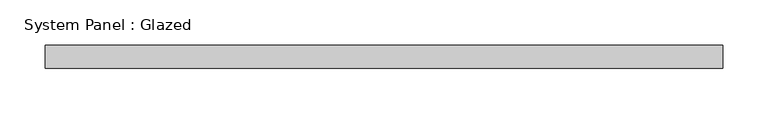
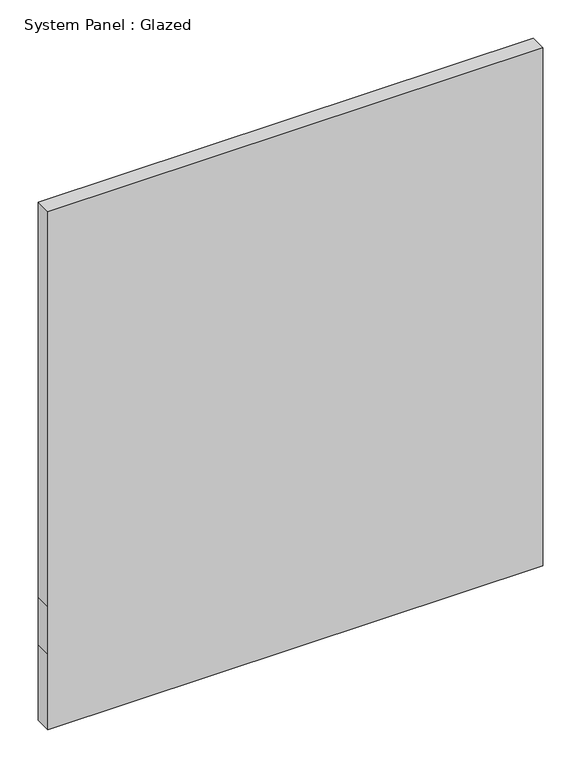
"""IFC4 building model written with IfcOpenShell, lengths in millimetres: plate geometry, System Panel : Glazed."""

from ifc_helpers import new_model, si_unit, frame, origin, place, context, project, spatial, polyline, outline, extrude, source, transform, mapped, element, save


def system_panel_glazed_1be55c4b(model_context):
    return source(origin(), model_context, "Body", "SweptSolid", [
        extrude(outline(polyline([(0.0, -374.65), (0.0, 374.65), (120.65, 374.65), (196.85, 374.65), (829.5094531, 374.65), (829.5094531, -374.65), (196.85, -374.65), (120.65, -374.65), (0.0, -374.65)])), frame((0.0, 19.05, 0.0), z_axis=(0.0, 1.0, 0.0), x_axis=(0.0, 0.0, 1.0)), (0.0, 0.0, 1.0), 25.4),
    ])


if __name__ == "__main__":
    model = new_model("IFC4")
    model_context = context("Model", 3, world=origin())
    ifc_project = project(units=[si_unit("LENGTHUNIT", "METRE", prefix="MILLI")], contexts=[model_context])
    site = spatial("IfcSite", under=ifc_project)
    building = spatial("IfcBuilding", under=site)
    placement = place(None, origin())
    system_panel_glazed_shape = system_panel_glazed_1be55c4b(model_context)
    element("IfcPlate", 1, ObjectType="System Panel : Glazed", at=placement, inside=building, context=model_context, shape_type="MappedRepresentation", body=[
        mapped(system_panel_glazed_shape, transform((0.0, 0.0, 0.0), x_axis=(1.0, 0.0, 0.0), y_axis=(0.0, 1.0, 0.0), z_axis=(0.0, 0.0, 1.0))),
    ])
    save(model, "model.ifc")

# Revit data of these elements
# Type "System Panel : Glazed"
#   Construction Type Id = "GSP4R"
#   Analytic Construction = "1/8 in Pilkington single glazing"
#   Visual Light Transmittance = 0.9
#   Solar Heat Gain Coefficient = 0.86
#   Heat Transfer Coefficient (U) = 1.18115 BTU/(h·ft²·°F)
#   Define Thermal Properties by = 1
# Element 1 (IfcPlate, "System Panel : Glazed")
#   Materials on its faces: "Glass"
# Materials
#   "Glass": class "Glass", colour RGB 0 128 192, transparency 0.75, Description = "Soda Lime Glass", Cost = 0
